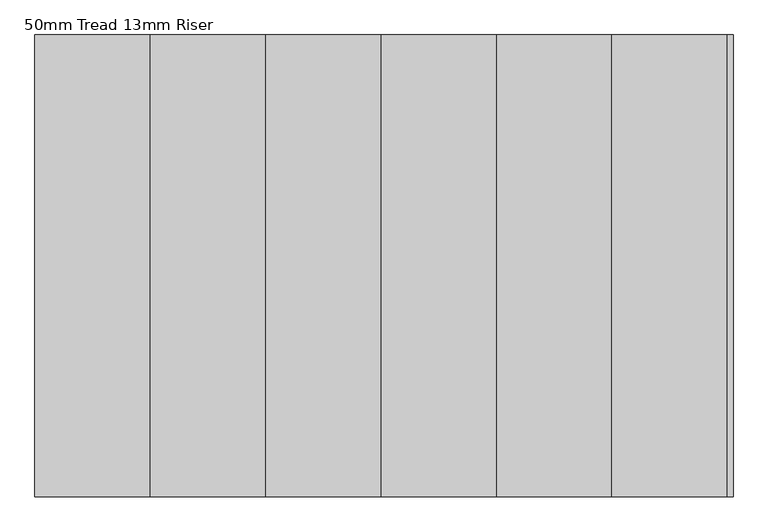
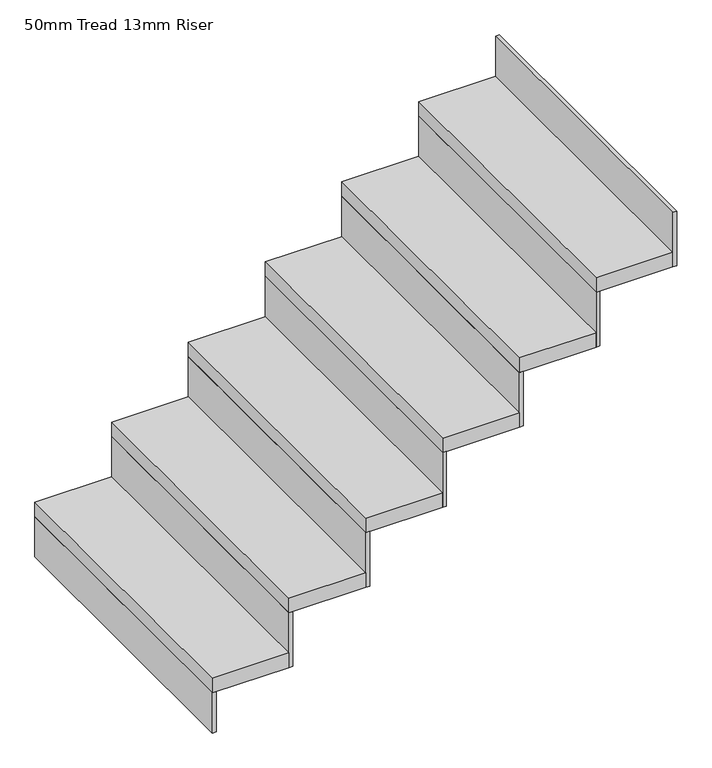
"""IFC4 building model written with IfcOpenShell, lengths in millimetres: stair flight geometry, 50mm Tread 13mm Riser."""

from ifc_helpers import new_model, si_unit, frame, origin, place, context, project, spatial, polyline, outline, extrude, source, transform, mapped, element, save


def stair_flight_50mm_tread_13mm_riser_0f073b0c(model_context):
    return source(origin(), model_context, "Body", "SweptSolid", [
        extrude(outline(polyline([(-11979.6794909, -2507.9876321), (-11992.1794909, -2507.9876321), (-11992.1794909, -1507.9618509), (-11979.6794909, -1507.9618509), (-11979.6794909, -2507.9876321)])), frame((0.0, 0.0, 3200.4), z_axis=(0.0, 0.0, 1.0), x_axis=(1.0, 0.0, 0.0)), (0.0, 0.0, 1.0), 138.2588235),
        extrude(outline(polyline([(-11742.1794909, -1507.9618509), (-11742.1794909, -2507.9876321), (-11992.1794909, -2507.9876321), (-11992.1794909, -1507.9618509), (-11742.1794909, -1507.9618509)])), frame((0.0, 0.0, 3338.6588235), z_axis=(0.0, 0.0, 1.0), x_axis=(1.0, 0.0, 0.0)), (0.0, 0.0, 1.0), 50.0),
        extrude(outline(polyline([(-11729.6794909, -2507.9876321), (-11742.1794909, -2507.9876321), (-11742.1794909, -1507.9618509), (-11729.6794909, -1507.9618509), (-11729.6794909, -2507.9876321)])), frame((0.0, 0.0, 3338.6588235), z_axis=(0.0, 0.0, 1.0), x_axis=(1.0, 0.0, 0.0)), (0.0, 0.0, 1.0), 188.2588235),
        extrude(outline(polyline([(-11492.1794909, -1507.9618509), (-11492.1794909, -2507.9876321), (-11742.1794909, -2507.9876321), (-11742.1794909, -1507.9618509), (-11492.1794909, -1507.9618509)])), frame((0.0, 0.0, 3526.9176471), z_axis=(0.0, 0.0, 1.0), x_axis=(1.0, 0.0, 0.0)), (0.0, 0.0, 1.0), 50.0),
        extrude(outline(polyline([(-11479.6794909, -2507.9876321), (-11492.1794909, -2507.9876321), (-11492.1794909, -1507.9618509), (-11479.6794909, -1507.9618509), (-11479.6794909, -2507.9876321)])), frame((0.0, 0.0, 3526.9176471), z_axis=(0.0, 0.0, 1.0), x_axis=(1.0, 0.0, 0.0)), (0.0, 0.0, 1.0), 188.2588235),
        extrude(outline(polyline([(-11242.1794909, -1507.9618509), (-11242.1794909, -2507.9876321), (-11492.1794909, -2507.9876321), (-11492.1794909, -1507.9618509), (-11242.1794909, -1507.9618509)])), frame((0.0, 0.0, 3715.1764706), z_axis=(0.0, 0.0, 1.0), x_axis=(1.0, 0.0, 0.0)), (0.0, 0.0, 1.0), 50.0),
        extrude(outline(polyline([(-11229.6794909, -2507.9876321), (-11242.1794909, -2507.9876321), (-11242.1794909, -1507.9618509), (-11229.6794909, -1507.9618509), (-11229.6794909, -2507.9876321)])), frame((0.0, 0.0, 3715.1764706), z_axis=(0.0, 0.0, 1.0), x_axis=(1.0, 0.0, 0.0)), (0.0, 0.0, 1.0), 188.2588235),
        extrude(outline(polyline([(-10992.1794909, -1507.9618509), (-10992.1794909, -2507.9876321), (-11242.1794909, -2507.9876321), (-11242.1794909, -1507.9618509), (-10992.1794909, -1507.9618509)])), frame((0.0, 0.0, 3903.4352941), z_axis=(0.0, 0.0, 1.0), x_axis=(1.0, 0.0, 0.0)), (0.0, 0.0, 1.0), 50.0),
        extrude(outline(polyline([(-10979.6794909, -2507.9876321), (-10992.1794909, -2507.9876321), (-10992.1794909, -1507.9618509), (-10979.6794909, -1507.9618509), (-10979.6794909, -2507.9876321)])), frame((0.0, 0.0, 3903.4352941), z_axis=(0.0, 0.0, 1.0), x_axis=(1.0, 0.0, 0.0)), (0.0, 0.0, 1.0), 188.2588235),
        extrude(outline(polyline([(-10742.1794909, -1507.9618509), (-10742.1794909, -2507.9876321), (-10992.1794909, -2507.9876321), (-10992.1794909, -1507.9618509), (-10742.1794909, -1507.9618509)])), frame((0.0, 0.0, 4091.6941176), z_axis=(0.0, 0.0, 1.0), x_axis=(1.0, 0.0, 0.0)), (0.0, 0.0, 1.0), 50.0),
        extrude(outline(polyline([(-10729.6794909, -2507.9876321), (-10742.1794909, -2507.9876321), (-10742.1794909, -1507.9618509), (-10729.6794909, -1507.9618509), (-10729.6794909, -2507.9876321)])), frame((0.0, 0.0, 4091.6941176), z_axis=(0.0, 0.0, 1.0), x_axis=(1.0, 0.0, 0.0)), (0.0, 0.0, 1.0), 188.2588235),
        extrude(outline(polyline([(-10479.6794909, -2507.9876321), (-10492.1794909, -2507.9876321), (-10492.1794909, -1507.9618509), (-10479.6794909, -1507.9618509), (-10479.6794909, -2507.9876321)])), frame((0.0, 0.0, 4279.9529412), z_axis=(0.0, 0.0, 1.0), x_axis=(1.0, 0.0, 0.0)), (0.0, 0.0, 1.0), 188.2588235),
        extrude(outline(polyline([(-10492.1794909, -1507.9618509), (-10492.1794909, -2507.9876321), (-10742.1794909, -2507.9876321), (-10742.1794909, -1507.9618509), (-10492.1794909, -1507.9618509)])), frame((0.0, 0.0, 4279.9529412), z_axis=(0.0, 0.0, 1.0), x_axis=(1.0, 0.0, 0.0)), (0.0, 0.0, 1.0), 50.0),
    ])


if __name__ == "__main__":
    model = new_model("IFC4")
    model_context = context("Model", 3, world=origin())
    ifc_project = project(units=[si_unit("LENGTHUNIT", "METRE", prefix="MILLI")], contexts=[model_context])
    site = spatial("IfcSite", under=ifc_project)
    building = spatial("IfcBuilding", under=site)
    placement = place(None, origin())
    stair_flight_50mm_tread_13mm_riser_shape = stair_flight_50mm_tread_13mm_riser_0f073b0c(model_context)
    element("IfcStairFlight", 1, ObjectType="50mm Tread 13mm Riser", at=placement, inside=building, context=model_context, shape_type="MappedRepresentation", body=[
        mapped(stair_flight_50mm_tread_13mm_riser_shape, transform((0.0, 0.0, 0.0), x_axis=(1.0, 0.0, 0.0), y_axis=(0.0, 1.0, 0.0), z_axis=(0.0, 0.0, 1.0))),
    ])
    save(model, "model.ifc")
